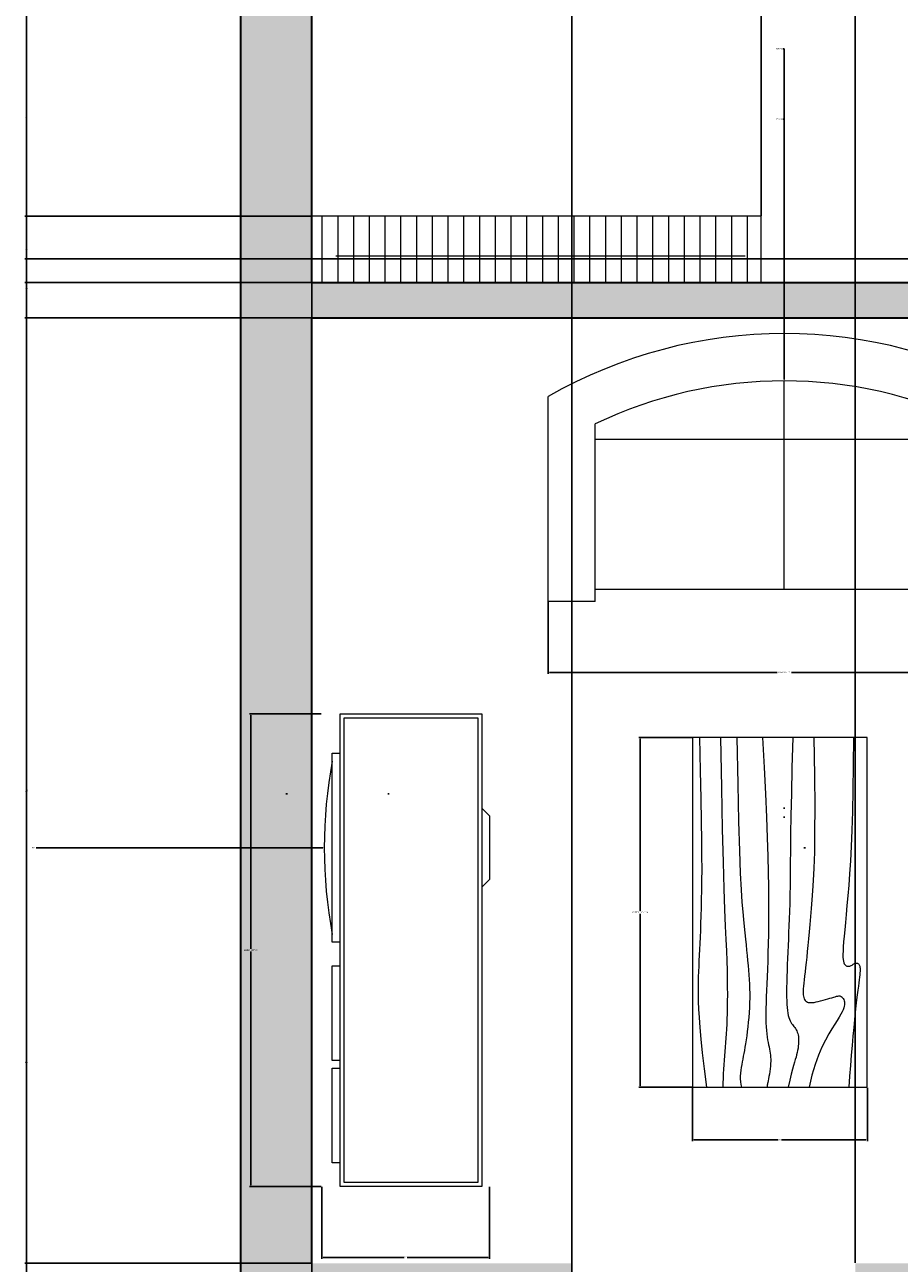
# Model space of a CAD drawing. Units: inches. Extents: x 1839 to 2285, y 722 to 1311.
# Tile 4 of 7: x 1870 to 1981, y 1018 to 1175. Entities that reach past the tile are written whole.
import ezdxf

# ---------------------------------------------------------------- set-up
doc = ezdxf.new("R2010")
doc.units = ezdxf.units.IN
for name, color, linetype, lineweight in [('A-ANNO-DIMS', 2, 'Continuous', 18), ('A-FLOR-CASE', 8, 'Continuous', 18), ('A-FLOR-PATT', 8, 'Continuous', 13), ('A-FURN', 8, 'Continuous', 18), ('A-WALL', 7, 'Continuous', 35)]:
    doc.layers.add(name, color=color, linetype=linetype, lineweight=lineweight)
doc.layers.add('A-WALL-PATT', color=18, linetype='Continuous', lineweight=13, true_color=0x000000)
doc.styles.get("Standard").update_dxf_attribs({"font": 'arial.ttf'})
doc.dimstyles.get("Standard").update_dxf_attribs({"dimtxt": 0.18, "dimasz": 0.18, "dimexe": 0.18, "dimexo": 0.0625, "dimgap": 0.09, "dimtad": 0, "dimtih": 1, "dimtoh": 1, "dimdec": 4, "dimzin": 0, "dimdsep": 46, "dimtxsty": 'Standard', "dimcen": 0.09, "dimadec": 0, "dimazin": 0, "dimtfac": 1, "dimtdec": 4, "dimtofl": 0, "dimtmove": 0, "dimatfit": 3, "dimfxl": 1, "dimtolj": 1, "dimtzin": 0, "dimarcsym": 0})

# ---------------------------------------------------------------- blocks, each defined once
blk = doc.blocks.new('Sofa - Roundback Loveseat 5 ft.')
for p, q in [((0, -32.44198), (0, -5.99998)), ((-24, -33.99998), (-24, -11.46958)), ((24.00004, -33.99998), (24.00004, -11.46958)), ((-23.9998, -13.38178), (23.99986, -13.38178)), ((-24, -32.44198), (24.00004, -32.44198))]:
    blk.add_line(p, q)
for points in [[(-24, -33.99998), (-30, -33.99998), (-30, -7.99998)], [(30.00004, -7.99998), (30.00004, -33.99998), (24.00004, -33.99998)]]:
    blk.add_lwpolyline(points)
for centre, radius, start, end in [((0, -60.24998), 60.24998, 60.13715, 119.8628), ((0, -61.38438), 55.38444, 64.32083, 115.6792)]:
    blk.add_arc(centre, radius, start, end)
blk = doc.blocks.new('Entertainment Center')
for p, q in [((-4, 0), (-5, -1)), ((4, 0), (-4, 0)), ((5, -1), (4, 0)), ((-17, -19), (-17, -1)), ((-17, -1), (43, -1)), ((-16.5, -18.5), (-16.5, -1.5)), ((-16.5, -1.5), (42.5, -1.5)), ((42.5, -1.5), (42.5, -18.5)), ((43, -1), (43, -19)), ((42.5, -18.5), (-16.5, -18.5)), ((43, -19), (-17, -19)), ((-12, -20), (-12, -19)), ((12, -20), (-12, -20)), ((12, -19), (12, -20)), ((15, -20), (15, -19)), ((27, -20), (15, -20)), ((27, -19), (27, -20)), ((28, -20), (28, -19)), ((40, -20), (28, -20)), ((40, -19), (40, -20))]:
    blk.add_line(p, q)
blk.add_arc((0, 40), 61, 259.6111, 280.3889)
blk = doc.blocks.new('Table - Rectangular Woodgrain 60 x 30 in.')
for p, q in [((0, 0), (0, -30)), ((60, 0), (0, 0)), ((60, -30), (60, 0)), ((0, -30), (60, -30))]:
    blk.add_line(p, q)
for points in [[(0, -2.4), (4.8155, -2.418), (9.0302, -2.4688), (12.709, -2.5477), (15.9167, -2.65), (18.7181, -2.7711), (21.1781, -2.9063), (23.3616, -3.0508), (25.3333, -3.2), (27.1477, -3.3495), (28.8172, -3.4958), (30.3437, -3.636), (31.7291, -3.7667), (32.9756, -3.8849), (34.0849, -3.9875), (35.059, -4.0714), (35.9, -4.1334), (36.6114, -4.1711), (37.2041, -4.1854), (37.6906, -4.1779), (38.0833, -4.15), (38.3948, -4.1034), (38.6375, -4.0396), (38.8239, -3.9602), (38.9666, -3.8667), (39.0764, -3.7608), (39.1573, -3.6448), (39.2116, -3.521), (39.2416, -3.3917), (39.2498, -3.2593), (39.2385, -3.1261), (39.21, -2.9944), (39.1666, -2.8667), (39.111, -2.7447), (39.0468, -2.6281), (38.978, -2.5163), (38.9083, -2.4083), (38.8418, -2.3035), (38.7823, -2.201), (38.7337, -2.1001), (38.7, -2), (38.6844, -1.9003), (38.6875, -1.8021), (38.7094, -1.707), (38.75, -1.6167), (38.8094, -1.5326), (38.8875, -1.4563), (38.9844, -1.3893), (39.1, -1.3333), (39.2351, -1.2896), (39.3937, -1.2583), (39.5804, -1.2396), (39.8, -1.2333), (40.057, -1.2396), (40.3562, -1.2583), (40.7023, -1.2896), (41.1, -1.3333), (41.5547, -1.3895), (42.0755, -1.4573), (42.6721, -1.5361), (43.3542, -1.625), (44.1316, -1.7233), (45.014, -1.8302), (46.0114, -1.9449), (47.1333, -2.0667), (48.3862, -2.1947), (49.7625, -2.3281), (51.2513, -2.4663), (52.8416, -2.6083), (54.5226, -2.7535), (56.2833, -2.9011), (58.1127, -3.0501), (60, -3.2)], [(0, -9.2), (6.5759, -9.0858), (11.9385, -9.0365), (16.2527, -9.0418), (19.6833, -9.0917), (22.3952, -9.1759), (24.5531, -9.2844), (26.322, -9.4069), (27.8666, -9.5333), (29.3241, -9.6553), (30.7203, -9.7719), (32.0532, -9.8837), (33.3208, -9.9917), (34.5213, -10.0965), (35.6526, -10.199), (36.7128, -10.2999), (37.7, -10.4), (38.6129, -10.4996), (39.4531, -10.5969), (40.223, -10.6895), (40.925, -10.775), (41.5613, -10.8512), (42.1344, -10.9156), (42.6465, -10.966), (43.1, -11), (43.4976, -11.0158), (43.8437, -11.0136), (44.143, -10.9942), (44.4, -10.9583), (44.6195, -10.9069), (44.8062, -10.8406), (44.9648, -10.7603), (45.1, -10.6667), (45.2155, -10.5598), (45.3114, -10.4365), (45.3871, -10.2929), (45.4416, -10.125), (45.4743, -9.929), (45.4844, -9.7011), (45.4709, -9.4371), (45.4333, -9.1333), (45.3716, -8.7883), (45.2896, -8.4104), (45.1919, -8.0107), (45.0833, -7.6), (44.9685, -7.1893), (44.8521, -6.7896), (44.7388, -6.4117), (44.6333, -6.0667), (44.54, -5.7628), (44.4614, -5.4979), (44.4001, -5.2675), (44.3583, -5.0667), (44.3384, -4.8909), (44.3427, -4.7354), (44.3736, -4.5956), (44.4333, -4.4667), (44.5236, -4.3453), (44.6427, -4.2333), (44.7884, -4.1339), (44.9583, -4.05), (45.1501, -3.9849), (45.3614, -3.9417), (45.59, -3.9234), (45.8333, -3.9333), (46.0915, -3.9749), (46.3734, -4.0531), (46.6906, -4.1736), (47.0542, -4.3417), (47.4756, -4.5629), (47.9661, -4.8427), (48.5372, -5.1866), (49.2, -5.6), (49.9676, -6.0844), (50.8594, -6.625), (51.8965, -7.2031), (53.1, -7.8), (54.491, -8.3969), (56.0906, -8.975), (57.9199, -9.5156), (60, -10)], [(0, -12.8), (5.1847, -12.9322), (9.6213, -13.0323), (13.3963, -13.1059), (16.5958, -13.1583), (19.3063, -13.1952), (21.614, -13.2219), (23.6054, -13.2439), (25.3666, -13.2667), (26.9728, -13.2947), (28.4531, -13.3281), (29.8256, -13.3663), (31.1083, -13.4083), (32.3191, -13.4535), (33.476, -13.501), (34.597, -13.5501), (35.7, -13.6), (36.7984, -13.6497), (37.8875, -13.6979), (38.9578, -13.743), (40, -13.7833), (41.0047, -13.8174), (41.9625, -13.8438), (42.864, -13.8607), (43.7, -13.8667), (44.4631, -13.8604), (45.1552, -13.8417), (45.7801, -13.8104), (46.3416, -13.7667), (46.8439, -13.7104), (47.2906, -13.6417), (47.6858, -13.5604), (48.0333, -13.4667), (48.3375, -13.3608), (48.6042, -13.2448), (48.8396, -13.121), (49.05, -12.9917), (49.2417, -12.8593), (49.4208, -12.7261), (49.5937, -12.5944), (49.7667, -12.4667), (49.9452, -12.3451), (50.1323, -12.2313), (50.3303, -12.1268), (50.5416, -12.0333), (50.7686, -11.9524), (51.0135, -11.8854), (51.2788, -11.8341), (51.5666, -11.8), (51.8785, -11.7843), (52.2116, -11.7865), (52.562, -11.8059), (52.926, -11.8417), (53.2998, -11.8931), (53.6795, -11.9594), (54.0614, -12.0397), (54.4416, -12.1333), (54.8223, -12.2401), (55.2293, -12.3625), (55.6942, -12.5037), (56.2489, -12.6667), (56.9251, -12.8547), (57.7545, -13.0708), (58.7689, -13.3182), (60, -13.6)], [(0, -18), (5.124, -17.7273), (9.6609, -17.5057), (13.6705, -17.3303), (17.2125, -17.1958), (20.3467, -17.0973), (23.1328, -17.0297), (25.6307, -16.9878), (27.9, -16.9667), (29.9928, -16.9617), (31.9302, -16.9703), (33.7254, -16.9907), (35.3917, -17.0208), (36.9423, -17.0588), (38.3906, -17.1026), (39.7499, -17.1503), (41.0333, -17.2), (42.2519, -17.2496), (43.4073, -17.2969), (44.4986, -17.3395), (45.525, -17.375), (46.4858, -17.4012), (47.3802, -17.4156), (48.2074, -17.416), (48.9667, -17.4), (49.6583, -17.3662), (50.2872, -17.3167), (50.8595, -17.2547), (51.3812, -17.1833), (51.8584, -17.1057), (52.2971, -17.025), (52.7034, -16.9443), (53.0833, -16.8667), (53.443, -16.7951), (53.789, -16.7313), (54.128, -16.6768), (54.4666, -16.6334), (54.8115, -16.6024), (55.1693, -16.5854), (55.5465, -16.5841), (55.95, -16.6), (56.3828, -16.6337), (56.8346, -16.6823), (57.2915, -16.7418), (57.7396, -16.8084), (58.165, -16.878), (58.5539, -16.9469), (58.8924, -17.0111), (59.1666, -17.0667), (59.3679, -17.1107), (59.5078, -17.1438), (59.6032, -17.1675), (59.6708, -17.1833), (59.7275, -17.193), (59.7901, -17.1979), (59.8753, -17.1998), (60, -17.2)], [(0, -22.4), (8.0098, -22.2501), (14.4094, -22.1011), (19.4168, -21.9535), (23.25, -21.8083), (26.1269, -21.6663), (28.2656, -21.5281), (29.884, -21.3947), (31.2, -21.2667), (32.3967, -21.1448), (33.5172, -21.0292), (34.5697, -20.9198), (35.5625, -20.8167), (36.5037, -20.7198), (37.4015, -20.6292), (38.2642, -20.5448), (39.1, -20.4667), (39.9164, -20.3951), (40.7187, -20.3313), (41.5117, -20.2768), (42.3, -20.2333), (43.0883, -20.2024), (43.8812, -20.1854), (44.6836, -20.1841), (45.5, -20.2), (46.3328, -20.234), (47.1747, -20.2844), (48.0163, -20.3488), (48.8479, -20.425), (49.66, -20.5106), (50.4429, -20.6031), (51.1872, -20.7004), (51.8833, -20.8), (52.5246, -20.8999), (53.1166, -20.9995), (53.6681, -21.0983), (54.1875, -21.1958), (54.6834, -21.2919), (55.1646, -21.3859), (55.6394, -21.4777), (56.1167, -21.5667), (56.6028, -21.6515), (57.0961, -21.7266), (57.5929, -21.7852), (58.0896, -21.8208), (58.5823, -21.8268), (59.0674, -21.7964), (59.5412, -21.723), (60, -21.6)], [(0, -25.2), (8.6355, -25.0504), (15.7026, -24.9031), (21.4049, -24.7606), (25.9458, -24.625), (29.529, -24.4988), (32.3578, -24.3844), (34.6359, -24.284), (36.5667, -24.2), (38.3213, -24.1341), (39.9417, -24.0854), (41.437, -24.0523), (42.8167, -24.0333), (44.0901, -24.0268), (45.2667, -24.0313), (46.3557, -24.0451), (47.3667, -24.0667), (48.309, -24.0947), (49.1928, -24.1287), (50.0284, -24.168), (50.826, -24.2125), (51.5959, -24.2617), (52.3483, -24.3151), (53.0935, -24.3725), (53.8417, -24.4334), (54.6009, -24.497), (55.3699, -24.561), (56.1454, -24.6226), (56.9239, -24.6792), (57.7021, -24.7279), (58.4764, -24.7662), (59.2435, -24.7911), (60, -24.8)], [(0, -28.8), (5.6867, -28.6681), (10.45, -28.5698), (14.407, -28.5012), (17.675, -28.4584), (20.3711, -28.4374), (22.6125, -28.4344), (24.5164, -28.4455), (26.2, -28.4667), (27.762, -28.4947), (29.2276, -28.5281), (30.6033, -28.5663), (31.8958, -28.6084), (33.1118, -28.6535), (34.2578, -28.7011), (35.3405, -28.7501), (36.3666, -28.8), (37.3443, -28.8497), (38.288, -28.8974), (39.2137, -28.9412), (40.1375, -28.9792), (41.0753, -29.0093), (42.0432, -29.0297), (43.0572, -29.0384), (44.1333, -29.0333), (45.2936, -29.0114), (46.5843, -28.9641), (48.0579, -28.8816), (49.7666, -28.7542), (51.7629, -28.5721), (54.0989, -28.3255), (56.8272, -28.0048), (60, -27.6)]]:
    blk.add_lwpolyline(points)
blk = doc.blocks.new('*D27')
at = {"layer": 'A-ANNO-DIMS', "color": 0, "lineweight": -2, "transparency": 16777216}
for p, q in [((1936.67, 1101.77), (1936.67, 1092.65)), ((1996.67, 1101.77), (1996.67, 1092.65)), ((1936.85, 1092.83), (1965.76, 1092.83)), ((1996.49, 1092.83), (1967.59, 1092.83))]:
    blk.add_line(p, q, dxfattribs=at)
at = {"layer": 'A-ANNO-DIMS', "color": 0, "transparency": 16777216}
for points in [[(1936.85, 1092.86), (1936.85, 1092.8), (1936.67, 1092.83)], [(1996.49, 1092.86), (1996.49, 1092.8), (1996.67, 1092.83)]]:
    blk.add_solid(points, dxfattribs=at)
at = {"layer": 'Defpoints', "color": 0, "transparency": 16777216}
for p in [(1936.67, 1101.83), (1996.67, 1101.83), (1996.67, 1092.83)]:
    blk.add_point(p, dxfattribs=at)
at = {"layer": 'A-ANNO-DIMS', "color": 0, "transparency": 16777216, "insert": (1966.67, 1092.83), "char_height": 0.18, "attachment_point": 5}
blk.add_mtext('\\A1;LOVESEAT 60', dxfattribs=at)
blk = doc.blocks.new('*D31')
at = {"layer": 'A-ANNO-DIMS', "color": 0, "lineweight": -2, "transparency": 16777216}
for p, q in [((1907.87, 1087.57), (1898.75, 1087.57)), ((1898.93, 1087.39), (1898.93, 1057.75)), ((1898.93, 1027.75), (1898.93, 1057.39)), ((1907.87, 1027.57), (1898.75, 1027.57))]:
    blk.add_line(p, q, dxfattribs=at)
at = {"layer": 'A-ANNO-DIMS', "color": 0, "transparency": 16777216}
for points in [[(1898.9, 1087.39), (1898.96, 1087.39), (1898.93, 1087.57)], [(1898.9, 1027.75), (1898.96, 1027.75), (1898.93, 1027.57)]]:
    blk.add_solid(points, dxfattribs=at)
at = {"layer": 'Defpoints', "color": 0, "transparency": 16777216}
for p in [(1907.93, 1087.57), (1898.93, 1027.57), (1907.93, 1027.57)]:
    blk.add_point(p, dxfattribs=at)
at = {"layer": 'A-ANNO-DIMS', "color": 0, "transparency": 16777216, "insert": (1898.93, 1057.57), "char_height": 0.18, "attachment_point": 5}
blk.add_mtext('\\A1;MEDIA UNIT 60', dxfattribs=at)
blk = doc.blocks.new('*D32')
at = {"layer": 'A-ANNO-DIMS', "color": 0, "lineweight": -2, "transparency": 16777216}
for p, q in [((1907.93, 1027.51), (1907.93, 1018.39)), ((1929.26, 1027.51), (1929.26, 1018.39)), ((1908.11, 1018.57), (1918.39, 1018.57)), ((1929.08, 1018.57), (1918.8, 1018.57))]:
    blk.add_line(p, q, dxfattribs=at)
at = {"layer": 'A-ANNO-DIMS', "color": 0, "transparency": 16777216}
for points in [[(1908.11, 1018.6), (1908.11, 1018.54), (1907.93, 1018.57)], [(1929.08, 1018.6), (1929.08, 1018.54), (1929.26, 1018.57)]]:
    blk.add_solid(points, dxfattribs=at)
at = {"layer": 'Defpoints', "color": 0, "transparency": 16777216}
for p in [(1907.93, 1027.57), (1929.26, 1027.57), (1929.26, 1018.57)]:
    blk.add_point(p, dxfattribs=at)
at = {"layer": 'A-ANNO-DIMS', "color": 0, "transparency": 16777216, "insert": (1918.6, 1018.57), "char_height": 0.18, "attachment_point": 5}
blk.add_mtext('\\A1;21', dxfattribs=at)
blk = doc.blocks.new('*D33')
at = {"layer": 'A-ANNO-DIMS', "color": 0, "lineweight": -2, "transparency": 16777216}
for p, q in [((1954.96, 1084.56), (1948.19, 1084.56)), ((1948.37, 1084.38), (1948.37, 1062.54)), ((1948.37, 1040.35), (1948.37, 1062.18)), ((1954.96, 1040.17), (1948.19, 1040.17))]:
    blk.add_line(p, q, dxfattribs=at)
at = {"layer": 'A-ANNO-DIMS', "color": 0, "transparency": 16777216}
for points in [[(1948.34, 1084.38), (1948.4, 1084.38), (1948.37, 1084.56)], [(1948.34, 1040.35), (1948.4, 1040.35), (1948.37, 1040.17)]]:
    blk.add_solid(points, dxfattribs=at)
at = {"layer": 'Defpoints', "color": 0, "transparency": 16777216}
for p in [(1955.02, 1084.56), (1948.37, 1040.17), (1955.02, 1040.17)]:
    blk.add_point(p, dxfattribs=at)
at = {"layer": 'A-ANNO-DIMS', "color": 0, "transparency": 16777216, "insert": (1948.37, 1062.36), "char_height": 0.18, "attachment_point": 5}
blk.add_mtext('\\A1;COFFEE TABLE 44', dxfattribs=at)
blk = doc.blocks.new('*D34')
at = {"layer": 'A-ANNO-DIMS', "color": 0, "lineweight": -2, "transparency": 16777216}
for p, q in [((1955.02, 1040.11), (1955.02, 1033.33)), ((1977.22, 1040.11), (1977.22, 1033.33)), ((1955.2, 1033.51), (1965.9, 1033.51)), ((1977.04, 1033.51), (1966.34, 1033.51))]:
    blk.add_line(p, q, dxfattribs=at)
at = {"layer": 'A-ANNO-DIMS', "color": 0, "transparency": 16777216}
for points in [[(1955.2, 1033.54), (1955.2, 1033.48), (1955.02, 1033.51)], [(1977.04, 1033.54), (1977.04, 1033.48), (1977.22, 1033.51)]]:
    blk.add_solid(points, dxfattribs=at)
at = {"layer": 'Defpoints', "color": 0, "transparency": 16777216}
for p in [(1955.02, 1040.17), (1977.22, 1040.17), (1977.22, 1033.51)]:
    blk.add_point(p, dxfattribs=at)
at = {"layer": 'A-ANNO-DIMS', "color": 0, "transparency": 16777216, "insert": (1966.12, 1033.51), "char_height": 0.18, "attachment_point": 5}
blk.add_mtext('\\A1;22', dxfattribs=at)
blk = doc.blocks.new('*D42')
at = {"layer": 'A-ANNO-DIMS', "color": 0, "lineweight": -2, "transparency": 16777216}
for p, q in [((1897.61, 1283.33), (1870.25, 1283.33)), ((1870.43, 1283.15), (1870.43, 1043.51)), ((1870.43, 803.51), (1870.43, 1043.15)), ((1897.61, 803.33), (1870.25, 803.33))]:
    blk.add_line(p, q, dxfattribs=at)
at = {"layer": 'A-ANNO-DIMS', "color": 0, "transparency": 16777216}
for points in [[(1870.4, 1283.15), (1870.46, 1283.15), (1870.43, 1283.33)], [(1870.4, 803.51), (1870.46, 803.51), (1870.43, 803.33)]]:
    blk.add_solid(points, dxfattribs=at)
at = {"layer": 'Defpoints', "color": 0, "transparency": 16777216}
for p in [(1870.43, 1283.33), (1897.68, 1283.33), (1897.68, 803.33)]:
    blk.add_point(p, dxfattribs=at)
at = {"layer": 'A-ANNO-DIMS', "color": 0, "transparency": 16777216, "insert": (1870.43, 1043.33), "char_height": 0.18, "attachment_point": 5}
blk.add_mtext('\\A1;480', dxfattribs=at)
blk = doc.blocks.new('*D43')
at = {"layer": 'A-ANNO-DIMS', "color": 0, "lineweight": -2, "transparency": 16777216}
for p, q in [((2050.68, 1145.27), (2050.68, 722.34)), ((1906.68, 1142.27), (1906.68, 722.34)), ((1906.86, 722.52), (1978.4, 722.52)), ((2050.5, 722.52), (1978.96, 722.52))]:
    blk.add_line(p, q, dxfattribs=at)
at = {"layer": 'A-ANNO-DIMS', "color": 0, "transparency": 16777216}
for points in [[(1906.86, 722.55), (1906.86, 722.49), (1906.68, 722.52)], [(2050.5, 722.55), (2050.5, 722.49), (2050.68, 722.52)]]:
    blk.add_solid(points, dxfattribs=at)
at = {"layer": 'Defpoints', "color": 0, "transparency": 16777216}
for p in [(2050.68, 1145.33), (1906.68, 1142.33), (2050.68, 722.52)]:
    blk.add_point(p, dxfattribs=at)
at = {"layer": 'A-ANNO-DIMS', "color": 0, "transparency": 16777216, "insert": (1978.68, 722.52), "char_height": 0.18, "attachment_point": 5}
blk.add_mtext('\\A1;144', dxfattribs=at)
blk = doc.blocks.new('*D48')
at = {"layer": 'A-ANNO-DIMS', "color": 0, "lineweight": -2, "transparency": 16777216}
for p, q in [((1906.61, 1137.83), (1870.25, 1137.83)), ((1870.43, 1137.65), (1870.43, 1078.01)), ((1870.43, 1018.01), (1870.43, 1077.65)), ((1906.61, 1017.83), (1870.25, 1017.83))]:
    blk.add_line(p, q, dxfattribs=at)
at = {"layer": 'A-ANNO-DIMS', "color": 0, "transparency": 16777216}
for points in [[(1870.4, 1137.65), (1870.46, 1137.65), (1870.43, 1137.83)], [(1870.4, 1018.01), (1870.46, 1018.01), (1870.43, 1017.83)]]:
    blk.add_solid(points, dxfattribs=at)
at = {"layer": 'Defpoints', "color": 0, "transparency": 16777216}
for p in [(1870.43, 1137.83), (1906.68, 1137.83), (1906.68, 1017.83)]:
    blk.add_point(p, dxfattribs=at)
at = {"layer": 'A-ANNO-DIMS', "color": 0, "transparency": 16777216, "insert": (1870.43, 1077.83), "char_height": 0.18, "attachment_point": 5}
blk.add_mtext('\\A1;120', dxfattribs=at)
blk = doc.blocks.new('*D66')
at = {"layer": 'A-ANNO-DIMS', "color": 0, "lineweight": -2, "transparency": 16777216}
for p, q in [((1975.68, 1017.89), (1975.68, 1310.76)), ((1975.86, 1310.58), (1999.77, 1310.58)), ((2024.48, 1310.58), (2000.57, 1310.58)), ((2024.66, 1017.89), (2024.66, 1310.76))]:
    blk.add_line(p, q, dxfattribs=at)
at = {"layer": 'A-ANNO-DIMS', "color": 0, "transparency": 16777216}
for points in [[(1975.86, 1310.61), (1975.86, 1310.55), (1975.68, 1310.58)], [(2024.48, 1310.61), (2024.48, 1310.55), (2024.66, 1310.58)]]:
    blk.add_solid(points, dxfattribs=at)
at = {"layer": 'Defpoints', "color": 0, "transparency": 16777216}
for p in [(2024.66, 1310.58), (1975.68, 1017.83), (2024.66, 1017.83)]:
    blk.add_point(p, dxfattribs=at)
at = {"layer": 'A-ANNO-DIMS', "color": 0, "transparency": 16777216, "insert": (2000.17, 1310.58), "char_height": 0.18, "attachment_point": 5}
blk.add_mtext('\\A1;48.99', dxfattribs=at)
blk = doc.blocks.new('*D70')
at = {"layer": 'A-ANNO-DIMS', "color": 0, "lineweight": -2, "transparency": 16777216}
for p, q in [((2104.61, 1181.33), (1870.25, 1181.33)), ((1870.43, 1181.15), (1870.43, 1163.51)), ((1870.43, 1145.51), (1870.43, 1163.15)), ((2104.61, 1145.33), (1870.25, 1145.33))]:
    blk.add_line(p, q, dxfattribs=at)
at = {"layer": 'A-ANNO-DIMS', "color": 0, "transparency": 16777216}
for points in [[(1870.4, 1181.15), (1870.46, 1181.15), (1870.43, 1181.33)], [(1870.4, 1145.51), (1870.46, 1145.51), (1870.43, 1145.33)]]:
    blk.add_solid(points, dxfattribs=at)
at = {"layer": 'Defpoints', "color": 0, "transparency": 16777216}
for p in [(1870.43, 1181.33), (2104.68, 1181.33), (2104.68, 1145.33)]:
    blk.add_point(p, dxfattribs=at)
at = {"layer": 'A-ANNO-DIMS', "color": 0, "transparency": 16777216, "insert": (1870.43, 1163.33), "char_height": 0.18, "attachment_point": 5}
blk.add_mtext('\\A1;36', dxfattribs=at)
blk = doc.blocks.new('*D73')
at = {"layer": 'A-ANNO-DIMS', "color": 0, "lineweight": -2, "transparency": 16777216}
for p, q in [((1906.68, 1150.79), (1906.68, 1310.76)), ((1906.86, 1310.58), (1934.8, 1310.58)), ((1963.54, 1310.58), (1935.59, 1310.58)), ((1963.72, 1150.79), (1963.72, 1310.76))]:
    blk.add_line(p, q, dxfattribs=at)
at = {"layer": 'A-ANNO-DIMS', "color": 0, "transparency": 16777216}
for points in [[(1906.86, 1310.61), (1906.86, 1310.55), (1906.68, 1310.58)], [(1963.54, 1310.61), (1963.54, 1310.55), (1963.72, 1310.58)]]:
    blk.add_solid(points, dxfattribs=at)
at = {"layer": 'Defpoints', "color": 0, "transparency": 16777216}
for p in [(1963.72, 1310.58), (1906.68, 1150.73), (1963.72, 1150.73)]:
    blk.add_point(p, dxfattribs=at)
at = {"layer": 'A-ANNO-DIMS', "color": 0, "transparency": 16777216, "insert": (1935.2, 1310.58), "char_height": 0.18, "attachment_point": 5}
blk.add_mtext('\\A1;57.04', dxfattribs=at)
blk = doc.blocks.new('*D75')
at = {"layer": 'A-ANNO-DIMS', "color": 0, "lineweight": -2, "transparency": 16777216}
for p, q in [((1906.61, 1150.73), (1870.25, 1150.73)), ((1870.43, 1150.55), (1870.43, 1146.71)), ((1870.43, 1142.51), (1870.43, 1146.35)), ((1906.61, 1142.33), (1870.25, 1142.33))]:
    blk.add_line(p, q, dxfattribs=at)
at = {"layer": 'A-ANNO-DIMS', "color": 0, "transparency": 16777216}
for points in [[(1870.4, 1150.55), (1870.46, 1150.55), (1870.43, 1150.73)], [(1870.4, 1142.51), (1870.46, 1142.51), (1870.43, 1142.33)]]:
    blk.add_solid(points, dxfattribs=at)
at = {"layer": 'Defpoints', "color": 0, "transparency": 16777216}
for p in [(1870.43, 1150.73), (1906.68, 1150.73), (1906.68, 1142.33)]:
    blk.add_point(p, dxfattribs=at)
at = {"layer": 'A-ANNO-DIMS', "color": 0, "transparency": 16777216, "insert": (1870.43, 1146.53), "char_height": 0.18, "attachment_point": 5}
blk.add_mtext('\\A1;8.4', dxfattribs=at)
blk = doc.blocks.new('*D81')
at = {"layer": 'A-ANNO-DIMS', "color": 0, "lineweight": -2, "transparency": 16777216}
for p, q in [((1906.68, 1013.39), (1906.68, 1310.76)), ((1906.86, 1310.58), (1922.96, 1310.58)), ((1939.5, 1310.58), (1923.4, 1310.58)), ((1939.68, 1013.39), (1939.68, 1310.76))]:
    blk.add_line(p, q, dxfattribs=at)
at = {"layer": 'A-ANNO-DIMS', "color": 0, "transparency": 16777216}
for points in [[(1906.86, 1310.61), (1906.86, 1310.55), (1906.68, 1310.58)], [(1939.5, 1310.61), (1939.5, 1310.55), (1939.68, 1310.58)]]:
    blk.add_solid(points, dxfattribs=at)
at = {"layer": 'Defpoints', "color": 0, "transparency": 16777216}
for p in [(1939.68, 1310.58), (1906.68, 1013.33), (1939.68, 1013.33)]:
    blk.add_point(p, dxfattribs=at)
at = {"layer": 'A-ANNO-DIMS', "color": 0, "transparency": 16777216, "insert": (1923.18, 1310.58), "char_height": 0.18, "attachment_point": 5}
blk.add_mtext('\\A1;33', dxfattribs=at)
blk = doc.blocks.new('*D83')
at = {"layer": 'A-ANNO-DIMS', "color": 0, "lineweight": -2, "transparency": 16777216}
for p, q in [((2104.61, 1145.33), (1870.25, 1145.33)), ((1870.43, 1145.15), (1870.43, 1141.76)), ((1870.43, 1138.01), (1870.43, 1141.4)), ((2104.61, 1137.83), (1870.25, 1137.83))]:
    blk.add_line(p, q, dxfattribs=at)
at = {"layer": 'A-ANNO-DIMS', "color": 0, "transparency": 16777216}
for points in [[(1870.4, 1145.15), (1870.46, 1145.15), (1870.43, 1145.33)], [(1870.4, 1138.01), (1870.46, 1138.01), (1870.43, 1137.83)]]:
    blk.add_solid(points, dxfattribs=at)
at = {"layer": 'Defpoints', "color": 0, "transparency": 16777216}
for p in [(1870.43, 1145.33), (2104.68, 1145.33), (2104.68, 1137.83)]:
    blk.add_point(p, dxfattribs=at)
at = {"layer": 'A-ANNO-DIMS', "color": 0, "transparency": 16777216, "insert": (1870.43, 1141.58), "char_height": 0.18, "attachment_point": 5}
blk.add_mtext('\\A1;7.5', dxfattribs=at)
blk = doc.blocks.new('*D86')
at = {"layer": 'A-ANNO-DIMS', "color": 0, "lineweight": -2, "transparency": 16777216}
for p, q in [((1903.39, 1077.42), (1903.57, 1077.42)), ((1903.48, 1077.33), (1903.48, 1077.51)), ((2097.39, 1077.42), (2024.85, 1077.42))]:
    blk.add_line(p, q, dxfattribs=at)
at = {"layer": 'A-ANNO-DIMS', "color": 0, "transparency": 16777216}
blk.add_solid([(2024.85, 1077.45), (2024.85, 1077.39), (2024.67, 1077.42)], dxfattribs=at)
at = {"layer": 'Defpoints', "color": 0, "transparency": 16777216}
for p in [(1903.48, 1077.42), (2024.67, 1077.42)]:
    blk.add_point(p, dxfattribs=at)
at = {"layer": 'A-ANNO-DIMS', "color": 0, "transparency": 16777216, "insert": (2097.87, 1077.42), "char_height": 0.18, "attachment_point": 5}
blk.add_mtext('\\A1;R121.2', dxfattribs=at)
blk = doc.blocks.new('*D87')
at = {"layer": 'A-ANNO-DIMS', "color": 0, "lineweight": -2, "transparency": 16777216}
for p, q in [((1916.33, 1077.42), (1916.51, 1077.42)), ((1916.42, 1077.33), (1916.42, 1077.51)), ((2099.22, 1077.42), (2030.85, 1077.42))]:
    blk.add_line(p, q, dxfattribs=at)
at = {"layer": 'A-ANNO-DIMS', "color": 0, "transparency": 16777216}
blk.add_solid([(2030.85, 1077.45), (2030.85, 1077.39), (2030.67, 1077.42)], dxfattribs=at)
at = {"layer": 'Defpoints', "color": 0, "transparency": 16777216}
for p in [(1916.42, 1077.42), (2030.67, 1077.42)]:
    blk.add_point(p, dxfattribs=at)
at = {"layer": 'A-ANNO-DIMS', "color": 0, "transparency": 16777216, "insert": (2099.77, 1077.42), "char_height": 0.18, "attachment_point": 5}
blk.add_mtext('\\A1;R114.25', dxfattribs=at)
blk = doc.blocks.new('*D88')
at = {"layer": 'A-ANNO-DIMS', "color": 0, "lineweight": -2, "transparency": 16777216}
for p, q in [((1871.66, 1070.57), (1908.08, 1070.57)), ((1969.17, 1070.57), (1969.35, 1070.57)), ((1969.26, 1070.48), (1969.26, 1070.66))]:
    blk.add_line(p, q, dxfattribs=at)
at = {"layer": 'A-ANNO-DIMS', "color": 0, "transparency": 16777216}
blk.add_solid([(1908.08, 1070.6), (1908.08, 1070.54), (1908.26, 1070.57)], dxfattribs=at)
at = {"layer": 'Defpoints', "color": 0, "transparency": 16777216}
for p in [(1908.26, 1070.57), (1969.26, 1070.57)]:
    blk.add_point(p, dxfattribs=at)
at = {"layer": 'A-ANNO-DIMS', "color": 0, "transparency": 16777216, "insert": (1871.38, 1070.57), "char_height": 0.18, "attachment_point": 5}
blk.add_mtext('\\A1;R61', dxfattribs=at)
blk = doc.blocks.new('*D89')
at = {"layer": 'A-ANNO-DIMS', "color": 0, "lineweight": -2, "transparency": 16777216}
for p, q in [((1966.49, 1171.98), (1966.67, 1171.98)), ((1966.67, 1171.98), (1966.67, 1136.01)), ((1966.58, 1075.58), (1966.76, 1075.58)), ((1966.67, 1075.49), (1966.67, 1075.67))]:
    blk.add_line(p, q, dxfattribs=at)
at = {"layer": 'A-ANNO-DIMS', "color": 0, "transparency": 16777216}
blk.add_solid([(1966.7, 1136.01), (1966.64, 1136.01), (1966.67, 1135.83)], dxfattribs=at)
at = {"layer": 'Defpoints', "color": 0, "transparency": 16777216}
for p in [(1966.67, 1135.83), (1966.67, 1075.58)]:
    blk.add_point(p, dxfattribs=at)
at = {"layer": 'A-ANNO-DIMS', "color": 0, "transparency": 16777216, "insert": (1966.01, 1171.98), "char_height": 0.18, "attachment_point": 5}
blk.add_mtext('\\A1;R60.25', dxfattribs=at)
blk = doc.blocks.new('*D90')
at = {"layer": 'A-ANNO-DIMS', "color": 0, "lineweight": -2, "transparency": 16777216}
for p, q in [((1966.49, 1163.06), (1966.67, 1163.06)), ((1966.67, 1163.06), (1966.67, 1130.01)), ((1966.58, 1074.45), (1966.76, 1074.45)), ((1966.67, 1074.36), (1966.67, 1074.54))]:
    blk.add_line(p, q, dxfattribs=at)
at = {"layer": 'A-ANNO-DIMS', "color": 0, "transparency": 16777216}
blk.add_solid([(1966.7, 1130.01), (1966.64, 1130.01), (1966.67, 1129.83)], dxfattribs=at)
at = {"layer": 'Defpoints', "color": 0, "transparency": 16777216}
for p in [(1966.67, 1129.83), (1966.67, 1074.45)]:
    blk.add_point(p, dxfattribs=at)
at = {"layer": 'A-ANNO-DIMS', "color": 0, "transparency": 16777216, "insert": (1966.01, 1163.06), "char_height": 0.18, "attachment_point": 5}
blk.add_mtext('\\A1;R55.38', dxfattribs=at)

msp = doc.modelspace()

# ---------------------------------------------------------------- hatches: boundary and pattern name
at = {"layer": 'A-FLOR-PATT'}
h = msp.add_hatch(dxfattribs=at)
h.set_pattern_fill('ANSI31', color=256, scale=0.629921, angle=45, style=0)
h.paths.add_polyline_path([(1906.6771, 1142.3314), (1963.7186, 1142.3314), (1963.7186, 1150.7318), (1906.6771, 1150.7318)])
at = {"layer": 'A-WALL-PATT'}
h = msp.add_hatch(color=256, dxfattribs=at)
h.dxf.hatch_style = 1
h.paths.add_polyline_path([(1906.6771, 1274.3314), (1942.6771, 1274.3314), (1942.6771, 1283.3314), (1897.6771, 1283.3314), (1897.6771, 968.2107), (1906.6771, 968.2107), (1906.6771, 1013.3314), (1939.6771, 1013.3314), (1939.6771, 1017.8314), (1906.6771, 1017.8314), (1906.6771, 1137.8314), (2050.6771, 1137.8314), (2050.6771, 1142.3314), (1906.6771, 1142.3314)])
h.paths.add_polyline_path([(2064.0508, 1283.3314), (1978.6771, 1283.3314), (1978.6771, 1274.3314), (2050.6771, 1274.3314), (2050.6771, 1184.3314), (2055.1771, 1184.3314), (2055.1771, 1214.3314), (2058.1771, 1214.3314), (2058.1771, 1218.8314), (2055.1771, 1218.8314), (2055.1771, 1274.3314), (2064.0508, 1274.3314)])
h.paths.add_polyline_path([(2182.6416, 1283.3314), (2088.0508, 1283.3314), (2088.0508, 1274.3314), (2104.6771, 1274.3314), (2104.6771, 1218.8314), (2094.1771, 1218.8314), (2094.1771, 1214.3314), (2104.6771, 1214.3314), (2104.6771, 1184.3314), (2109.1771, 1184.3314), (2109.1771, 1274.3314), (2182.6416, 1274.3314)])
h.paths.add_polyline_path([(2257.6771, 1283.3314), (2218.6416, 1283.3314), (2218.6416, 1274.3314), (2248.6771, 1274.3314), (2248.6771, 1142.3314), (2186.4004, 1142.3314), (2109.1771, 1142.3314), (2109.1771, 1137.8314), (2248.6771, 1137.8314), (2248.6771, 1094.9086), (2257.6771, 1094.9086)])
h.paths.add_polyline_path([(2257.6771, 1058.9086), (2248.6771, 1058.9086), (2248.6771, 1017.8314), (2160.1771, 1017.8314), (2160.1771, 939.8314), (2164.6771, 939.8314), (2164.6771, 1013.3314), (2248.6771, 1013.3314), (2248.6771, 977.3314), (2248.6771, 950.4862), (2257.6771, 950.4862)])
h.paths.add_polyline_path([(2257.6771, 893.3314), (2248.6771, 893.3314), (2248.6771, 850.1143), (2190.4862, 850.1143), (2190.4862, 845.6143), (2248.6771, 845.6143), (2248.6771, 812.3314), (2100.5038, 812.3314), (2100.5038, 803.3314), (2257.6771, 803.3314)])
h.paths.add_polyline_path([(2257.6771, 926.4862), (2248.6771, 926.4862), (2248.6771, 897.8314), (2141.6642, 897.8314), (2141.6642, 893.3314), (2145.5038, 893.3314), (2145.5038, 812.3314), (2147.5038, 812.3314), (2147.5038, 845.6143), (2153.9854, 845.6143), (2153.9854, 850.1143), (2147.5038, 850.1143), (2147.5038, 893.3314), (2248.6771, 893.3314), (2257.6771, 893.3314)])
h.paths.add_polyline_path([(1906.6771, 893.3314), (1897.6771, 893.3314), (1897.6771, 803.3314), (2022.5038, 803.3314), (2022.5038, 812.3314), (1906.6771, 812.3314)])
h.paths.add_polyline_path([(2031.4676, 897.8314), (1981.6771, 897.8314), (1981.6771, 1013.3314), (2024.6642, 1013.3314), (2024.6642, 1017.8314), (1975.6771, 1017.8314), (1975.6771, 1013.3314), (1978.6771, 1013.3314), (1978.6771, 897.8314), (1906.6771, 897.8314), (1906.6771, 932.2107), (1897.6771, 932.2107), (1897.6771, 893.3314), (1906.6771, 893.3314), (2031.4676, 893.3314)])
h.paths.add_polyline_path([(2099.6642, 1017.8314), (2096.6642, 1017.8314), (2084.1956, 1017.8314), (2084.1956, 1013.3314), (2096.6642, 1013.3314), (2096.6642, 897.8314), (2085.6129, 897.8314), (2085.6129, 893.3314), (2102.6642, 893.3314), (2102.6642, 897.8314), (2099.6642, 897.8314)])

# ---------------------------------------------------------------- linework, layer by layer
at = {"layer": 'A-FLOR-CASE'}
for p, q in [((1963.7186, 1150.7318), (1906.6771, 1150.7318)), ((1906.6771, 1150.7318), (1906.6771, 1142.3314)), ((1963.7186, 1142.3314), (1963.7186, 1150.7318)), ((1909.7186, 1145.7055), (1961.7186, 1145.7055)), ((1906.6771, 1142.3314), (1963.7186, 1142.3314))]:
    msp.add_line(p, q, dxfattribs=at)
at = {"layer": 'A-WALL'}
for p, q in [((1906.6771, 1142.3314), (1906.6771, 1274.3314)), ((1906.6771, 1142.3314), (2055.1771, 1142.3314)), ((1906.6771, 1137.8314), (2055.1771, 1137.8314)), ((1906.6771, 1017.8314), (1906.6771, 1137.8314))]:
    msp.add_line(p, q, dxfattribs=at)
msp.add_lwpolyline([(2022.5038, 803.3314), (1897.6771, 803.3314), (1897.6771, 1283.3314), (2257.6771, 1283.3314), (2257.6771, 803.3314), (2100.5038, 803.3314)], dxfattribs=at)

# ---------------------------------------------------------------- block references
at = {"layer": 'A-FURN'}
msp.add_blockref('Sofa - Roundback Loveseat 5 ft.', (1966.6741, 1135.8314), dxfattribs=at)
at = {"layer": 'A-FURN', "rotation": 270}
msp.add_blockref('Entertainment Center', (1929.263, 1070.5724), dxfattribs=at)
at = {"layer": 'A-FURN', "xscale": 0.7397827504390865, "yscale": 0.7397827504390865, "zscale": 0.7397827504390865, "rotation": 270}
msp.add_blockref('Table - Rectangular Woodgrain 60 x 30 in.', (1977.2167, 1084.5551), dxfattribs=at)

# ---------------------------------------------------------------- dimensions: what is measured, and where the dimension line sits
at = {"layer": 'A-ANNO-DIMS'}
for base, p1, p2, override, picture, middle in [((1963.7186, 1310.5814), (1906.6771, 1150.7318), (1963.7186, 1150.7318), {"dimdec": 2, "dimlfac": 1, "dimrnd": 0, "dimzin": 0, "dimdsep": 46, "dimlunit": 2}, '*D73', (1935.1978, 1310.5814)), ((1939.6771, 1310.5814), (1906.6771, 1013.3314), (1939.6771, 1013.3314), {"dimdec": 0, "dimlfac": 1, "dimrnd": 0, "dimzin": 0, "dimdsep": 46, "dimlunit": 2}, '*D81', (1923.1771, 1310.5814)), ((2024.6642, 1310.5814), (1975.6771, 1017.8314), (2024.6642, 1017.8314), {"dimdec": 2, "dimlfac": 1, "dimrnd": 0, "dimzin": 0, "dimdsep": 46, "dimlunit": 2}, '*D66', (2000.1706, 1310.5814)), ((2050.6771, 722.516), (1906.6771, 1142.3314), (2050.6771, 1145.3314), {"dimdec": 0, "dimlfac": 1, "dimrnd": 0, "dimzin": 0, "dimdsep": 46, "dimlunit": 2}, '*D43', (1978.6771, 722.516)), ((1977.2167, 1033.5101), (1955.0232, 1040.1681), (1977.2167, 1040.1681), {"dimdec": 0, "dimlfac": 1, "dimrnd": 0, "dimzin": 0, "dimdsep": 46, "dimlunit": 2}, '*D34', (1966.1199, 1033.5101)), ((1929.263, 1018.5724), (1907.9297, 1027.5724), (1929.263, 1027.5724), {"dimdec": 0, "dimlfac": 1, "dimrnd": 0, "dimzin": 0, "dimdsep": 46, "dimlunit": 2}, '*D32', (1918.5963, 1018.5724))]:
    dim = msp.add_linear_dim(base=base, p1=p1, p2=p2, dimstyle='Standard', override=override, dxfattribs=at)
    dim.commit()
    dim.dimension.update_dxf_attribs({"geometry": picture, "text_midpoint": middle})
for base, p1, p2, override, picture, middle in [((1870.4271, 1283.3314), (1897.6771, 803.3314), (1897.6771, 1283.3314), {"dimdec": 0, "dimlfac": 1, "dimrnd": 0, "dimzin": 0, "dimdsep": 46, "dimlunit": 2}, '*D42', (1870.4271, 1043.3314)), ((1870.4271, 1181.3314), (2104.6771, 1145.3314), (2104.6771, 1181.3314), {"dimdec": 0, "dimlfac": 1, "dimrnd": 0, "dimzin": 0, "dimdsep": 46, "dimlunit": 2}, '*D70', (1870.4271, 1163.3314)), ((1870.4271, 1150.7318), (1906.6771, 1142.3314), (1906.6771, 1150.7318), {"dimdec": 1, "dimlfac": 1, "dimrnd": 0, "dimzin": 0, "dimdsep": 46, "dimlunit": 2}, '*D75', (1870.4271, 1146.5316)), ((1870.4271, 1145.3314), (2104.6771, 1137.8314), (2104.6771, 1145.3314), {"dimdec": 1, "dimlfac": 1, "dimrnd": 0, "dimzin": 0, "dimdsep": 46, "dimlunit": 2}, '*D83', (1870.4271, 1141.5814)), ((1870.4271, 1137.8314), (1906.6771, 1017.8314), (1906.6771, 1137.8314), {"dimdec": 0, "dimlfac": 1, "dimrnd": 0, "dimzin": 0, "dimdsep": 46, "dimlunit": 2}, '*D48', (1870.4271, 1077.8314))]:
    dim = msp.add_linear_dim(base=base, p1=p1, p2=p2, angle=90, dimstyle='Standard', override=override, dxfattribs=at)
    dim.commit()
    dim.dimension.update_dxf_attribs({"geometry": picture, "text_midpoint": middle})
for center, mpoint, override, picture, middle in [((1966.6741, 1075.5814), (1966.674, 1135.8314), {"dimdec": 2, "dimlfac": 1, "dimrnd": 0, "dimzin": 0, "dimdsep": 46, "dimlunit": 2}, '*D89', (1966.0134, 1171.9814)), ((1966.6741, 1074.447), (1966.674, 1129.8315), {"dimdec": 2, "dimlfac": 1, "dimrnd": 0, "dimzin": 0, "dimdsep": 46, "dimlunit": 2}, '*D90', (1966.0139, 1163.0621)), ((1903.4774, 1077.4214), (2024.6742, 1077.421), {"dimdec": 1, "dimlfac": 1, "dimrnd": 0, "dimzin": 0, "dimdsep": 46, "dimlunit": 2}, '*D86', (2097.3922, 1077.4208)), ((1916.4242, 1077.4214), (2030.6742, 1077.421), {"dimdec": 2, "dimlfac": 1, "dimrnd": 0, "dimzin": 0, "dimdsep": 46, "dimlunit": 2}, '*D87', (2099.2242, 1077.4208)), ((1969.263, 1070.5724), (1908.263, 1070.572), {"dimdec": 0, "dimlfac": 1, "dimrnd": 0, "dimzin": 0, "dimdsep": 46, "dimlunit": 2}, '*D88', (1871.663, 1070.5718))]:
    dim = msp.add_radius_dim(center=center, mpoint=mpoint, dimstyle='Standard', override=override, dxfattribs=at)
    dim.commit()
    dim.dimension.update_dxf_attribs({"geometry": picture, "text_midpoint": middle, "dimtype": 164})
dim = msp.add_linear_dim(base=(1996.6742, 1092.8314), p1=(1936.6741, 1101.8314), p2=(1996.6742, 1101.8314), text='LOVESEAT <>', dimstyle='Standard', override={"dimdec": 0, "dimlfac": 1, "dimrnd": 0, "dimzin": 0, "dimdsep": 46, "dimlunit": 2}, dxfattribs=at)
dim.commit()
dim.dimension.update_dxf_attribs({"geometry": '*D27', "text_midpoint": (1966.6741, 1092.8314)})
for base, p1, p2, text, picture, middle in [((1898.9297, 1027.5724), (1907.9297, 1087.5724), (1907.9297, 1027.5724), 'MEDIA UNIT <>', '*D31', (1898.9297, 1057.5724)), ((1948.3652, 1040.1681), (1955.0232, 1084.5551), (1955.0232, 1040.1681), 'COFFEE TABLE <>', '*D33', (1948.3652, 1062.3616))]:
    dim = msp.add_linear_dim(base=base, p1=p1, p2=p2, angle=270, text=text, dimstyle='Standard', override={"dimdec": 0, "dimlfac": 1, "dimrnd": 0, "dimzin": 0, "dimdsep": 46, "dimlunit": 2}, dxfattribs=at)
    dim.commit()
    dim.dimension.update_dxf_attribs({"geometry": picture, "text_midpoint": middle})

doc.saveas('drawing.dxf')
